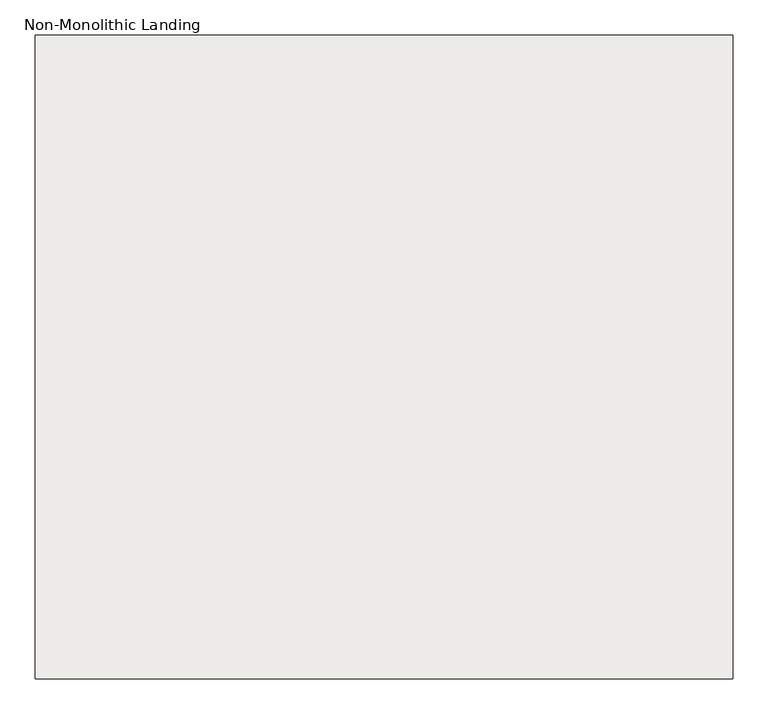
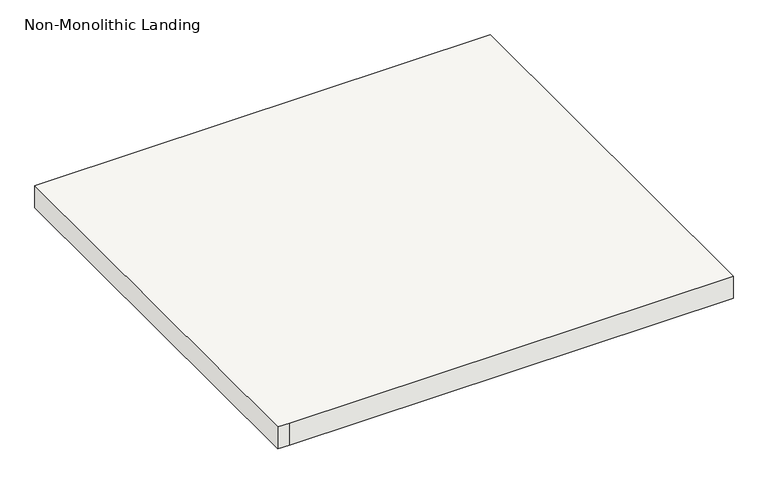
"""IFC4 building model written with IfcOpenShell, lengths in millimetres: slab geometry, Non-Monolithic Landing."""

from ifc_helpers import new_model, si_unit, origin, place, context, project, spatial, faceted_brep, source, transform, mapped, element, save


def non_monolithic_landing_70e0e3a4(model_context):
    return source(origin(), model_context, "Body", "Brep", [
        faceted_brep([(3609.7430349, 2997.8555142, 2060.7617647), (3609.7430349, 2972.4555142, 2035.3617647), (2695.3430349, 2972.4555142, 2035.3617647), (2695.3430349, 2997.8555142, 2060.7617647), (2644.5430349, 2997.8555142, 2079.8117647), (2619.1430349, 2997.8555142, 2079.8117647), (2619.1430349, 2083.4555142, 2079.8117647), (2644.5430349, 2083.4555142, 2079.8117647), (3609.7430349, 2083.4555142, 2079.8117647), (3609.7430349, 2997.8555142, 2079.8117647), (2695.3430349, 2972.4555142, 2029.0117647), (3609.7430349, 2972.4555142, 2029.0117647), (3609.7430349, 2083.4555142, 2029.0117647), (2644.5430349, 2083.4555142, 2029.0117647), (2619.1430349, 2083.4555142, 2029.0117647), (2619.1430349, 2997.8555142, 2029.0117647), (2644.5430349, 2997.8555142, 2029.0117647), (2695.3430349, 2997.8555142, 2029.0117647)], [[[0, 1, 2, 3]], [[4, 5, 6, 7, 8, 9]], [[10, 11, 12, 13, 14, 15, 16, 17]], [[11, 10, 2, 1]], [[10, 17, 3, 2]], [[4, 9, 0, 3, 17, 16]], [[5, 4, 16, 15]], [[6, 5, 15, 14]], [[7, 6, 14, 13]], [[8, 7, 13, 12]], [[9, 8, 12, 11, 1, 0]]]),
    ])


if __name__ == "__main__":
    model = new_model("IFC4")
    model_context = context("Model", 3, world=origin())
    ifc_project = project(units=[si_unit("LENGTHUNIT", "METRE", prefix="MILLI")], contexts=[model_context])
    site = spatial("IfcSite", under=ifc_project)
    building = spatial("IfcBuilding", under=site)
    placement = place(None, origin())
    non_monolithic_landing_shape = non_monolithic_landing_70e0e3a4(model_context)
    element("IfcSlab", 1, ObjectType="Non-Monolithic Landing", at=placement, inside=building, context=model_context, shape_type="MappedRepresentation", body=[
        mapped(non_monolithic_landing_shape, transform((0.0, 0.0, 0.0), x_axis=(1.0, 0.0, 0.0), y_axis=(0.0, 1.0, 0.0), z_axis=(0.0, 0.0, 1.0))),
    ])
    save(model, "model.ifc")
